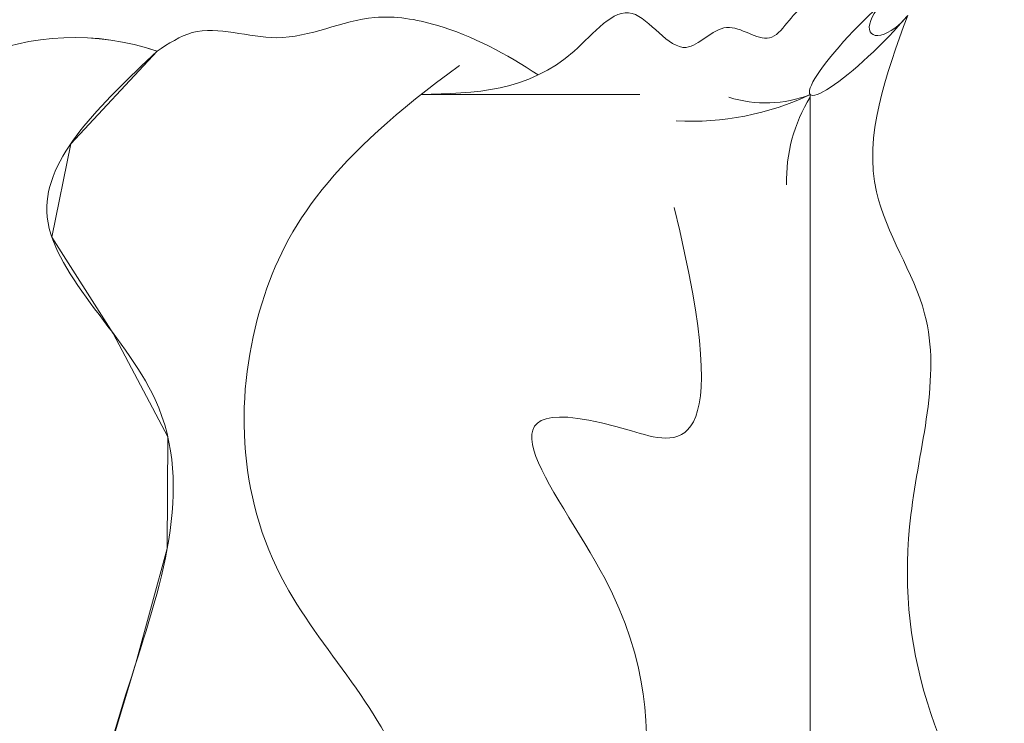
# Model space of a CAD drawing. Units: inches. Extents: x 2083 to 3317, y 1141 to 2115.
# Tile 10 of 256: x 2278 to 2324, y 1329 to 1361. Entities that reach past the tile are written whole.
import ezdxf

# ---------------------------------------------------------------- set-up
doc = ezdxf.new("R2010")
doc.units = ezdxf.units.IN
for name, color, linetype, lineweight in [('A-ANNO-DIMS', 2, 'Continuous', 18), ('A-FURN', 8, 'Continuous', 18), ('www.cadblocksfree.com', 7, 'Continuous', 9)]:
    doc.layers.add(name, color=color, linetype=linetype, lineweight=lineweight)
doc.layers.add('A-WALL-PATT', color=251, linetype='Continuous', lineweight=13, true_color=0x636466)
doc.styles.get("Standard").update_dxf_attribs({"font": 'arial.ttf'})
doc.dimstyles.new('ISO-25', dxfattribs={"dimtxt": 12, "dimasz": 12, "dimexe": 1.25, "dimexo": 0.625, "dimtad": 1, "dimlunit": 3, "dimtxsty": 'Standard', "dimcen": 2.5, "dimadec": 0, "dimazin": 0, "dimtfac": 1, "dimtmove": 0, "dimatfit": 3, "dimfxl": 1, "dimarcsym": 0})

# ---------------------------------------------------------------- blocks, each defined once
blk = doc.blocks.new('bed')
at = {"layer": 'www.cadblocksfree.com', "ltscale": 0.2}
for p, q in [((3426.379, 1399.908), (3426.379, 1410.814)), ((3363.387, 1391.414), (3426.379, 1391.414))]:
    blk.add_line(p, q, dxfattribs=at)
for centre, radius, start, end in [((3416.575, 1428.082), 12.646, 341.0268, 23.7782), ((3438.819, 1397.314), 13.768, 176.7525, 205.373), ((3432.135, 1393.639), 6.173, 162.6475, 201.1361), ((3422.111, 1384.801), 7.798, 58.0013, 91.6551)]:
    blk.add_arc(centre, radius, start, end, dxfattribs=at)
for centre, major_axis, ratio, start_param, end_param in [((3429.422, 1388.371), (-3.043, 3.043), 0.168252, 4.250342, 8.316029), ((3430.477, 1387.316), (-1.055, 1.055), 0.453532, 4.422107, 8.144264)]:
    blk.add_ellipse(centre, major_axis=major_axis, ratio=ratio, start_param=start_param, end_param=end_param, dxfattribs=at)
for points, knots in [([(3365.512, 1424.213), (3370.519, 1427.004), (3381.149, 1429.825), (3396.214, 1425.866), (3410.541, 1420.654), (3420.273, 1432.695), (3425.882, 1426.771), (3428.534, 1423.97)], [0.099185, 0.099185, 0.099185, 0.099185, 0.523647, 0.927087, 1.289918, 1.564439, 1.810555, 1.810555, 1.810555, 1.810555]), ([(3428.534, 1423.97), (3428.914, 1423.397), (3430.098, 1421.613), (3428.491, 1417.656), (3430.593, 1413.794), (3429.801, 1409.122), (3428.396, 1406.564), (3427.355, 1404.971)], [0, 0, 0, 0, 0.050513, 0.157399, 0.2842023, 0.3628173, 0.5066917, 0.5066917, 0.5066917, 0.5066917]), ([(3362.057, 1409.866), (3363.638, 1413.65), (3372.978, 1421.337), (3389.682, 1406.045), (3402.396, 1419.984), (3416.037, 1420.167), (3423.233, 1415.231), (3427.827, 1408.899)], [0.029901, 0.029901, 0.029901, 0.029901, 0.276967, 0.797115, 1.093669, 1.464666, 1.788489, 1.788489, 1.788489, 1.788489]), ([(3431.237, 1387.473), (3430.882, 1388.172), (3430.205, 1389.505), (3431.478, 1391.985), (3428.294, 1393.194), (3430.501, 1395.689), (3427.558, 1397.866), (3431.841, 1400.386), (3426.535, 1404.33), (3426.443, 1408.152), (3426.379, 1410.814)], [0, 0, 0, 0, 2.267059, 4.324559, 6.685584, 8.878641, 11.121502, 14.300359, 17.755284, 25.682856, 25.682856, 25.682856, 25.682856]), ([(3368.632, 1397.839), (3375.978, 1400.489), (3385.349, 1402.757), (3397.531, 1395.273), (3413.593, 1410.377), (3407.806, 1395.019), (3420.759, 1398.2)], [0.029901, 0.029901, 0.029901, 0.029901, 0.276967, 0.797115, 1.093669, 1.16836, 1.16836, 1.16836, 1.16836]), ([(3430.32, 1386.556), (3427.327, 1387.653), (3422.148, 1389.55), (3414.529, 1384.137), (3405.607, 1387.046), (3396.29, 1386.314), (3386.838, 1381.282), (3377.742, 1390.272), (3370.778, 1384.799), (3364.626, 1383.966), (3363.275, 1388.265), (3360.778, 1387.151), (3359.446, 1386.556)], [0, 0, 0, 0, 8.93042, 15.449194, 25.485629, 34.878505, 43.598887, 54.554403, 64.16647, 67.461673, 70.610457, 74.213583, 74.213583, 74.213583, 74.213583])]:
    blk.add_open_spline(points, degree=3, knots=knots, dxfattribs=at)
blk = doc.blocks.new('*D22')
at = {"layer": 'A-ANNO-DIMS', "color": 0, "lineweight": -2, "transparency": 16777216}
for p, q in [((2235.96, 1362.739), (2235.96, 1376.309)), ((2322.26, 1362.739), (2322.26, 1376.309)), ((2235.96, 1375.059), (2083.007, 1375.059)), ((2310.26, 1375.059), (2247.96, 1375.059))]:
    blk.add_line(p, q, dxfattribs=at)
at = {"layer": 'A-ANNO-DIMS', "color": 0, "transparency": 16777216}
for points in [[(2247.96, 1377.059), (2247.96, 1373.059), (2235.96, 1375.059)], [(2310.26, 1377.059), (2310.26, 1373.059), (2322.26, 1375.059)]]:
    blk.add_solid(points, dxfattribs=at)
at = {"layer": 'Defpoints', "color": 0, "transparency": 16777216}
for p in [(2235.96, 1375.059), (2235.96, 1362.114), (2322.26, 1362.114)]:
    blk.add_point(p, dxfattribs=at)
at = {"layer": 'A-ANNO-DIMS', "color": 0, "transparency": 16777216, "insert": (2153.483, 1381.889), "char_height": 12, "attachment_point": 5}
blk.add_mtext('BED 7\'-2 1/2" TYP.', dxfattribs=at)
blk = doc.blocks.new('*D23')
at = {"layer": 'A-ANNO-DIMS', "color": 0, "lineweight": -2, "transparency": 16777216}
for p, q in [((2335.205, 1362.114), (2335.205, 1476.472)), ((2322.885, 1362.114), (2336.455, 1362.114)), ((2335.205, 1306.473), (2335.205, 1350.114)), ((2322.885, 1294.473), (2336.455, 1294.473))]:
    blk.add_line(p, q, dxfattribs=at)
at = {"layer": 'A-ANNO-DIMS', "color": 0, "transparency": 16777216}
for points in [[(2333.205, 1350.114), (2337.205, 1350.114), (2335.205, 1362.114)], [(2333.205, 1306.473), (2337.205, 1306.473), (2335.205, 1294.473)]]:
    blk.add_solid(points, dxfattribs=at)
at = {"layer": 'Defpoints', "color": 0, "transparency": 16777216}
for p in [(2322.26, 1362.114), (2335.205, 1362.114), (2322.26, 1294.473)]:
    blk.add_point(p, dxfattribs=at)
at = {"layer": 'A-ANNO-DIMS', "color": 0, "transparency": 16777216, "insert": (2328.376, 1425.293), "char_height": 12, "attachment_point": 5, "rotation": 90}
blk.add_mtext('5\'-7 1/2" TYP.', dxfattribs=at)

msp = doc.modelspace()

# ---------------------------------------------------------------- hatches: boundary and pattern name
at = {"layer": 'A-WALL-PATT'}
h = msp.add_hatch(color=256, dxfattribs=at)
h.dxf.hatch_style = 1
h.paths.add_polyline_path([(3126.96, 2020.761), (2748.96, 2020.761), (2604.96, 2020.761), (2226.96, 2020.761), (2226.96, 1702.761), (2466.96, 1702.761), (2466.96, 1582.761), (2418.96, 1582.761), (2418.96, 1477.761), (2226.96, 1477.761), (2226.96, 1263.261), (2544.96, 1263.261), (2544.96, 1411.761), (2604.96, 1411.761), (2685.96, 1411.761), (2685.96, 1420.761), (2604.96, 1420.761), (2604.96, 1573.761), (2604.96, 1702.761), (2604.96, 2011.761), (2748.96, 2011.761), (2748.96, 1702.761), (2862.96, 1702.761), (2862.96, 1621.761), (2871.96, 1621.761), (2871.96, 1702.761), (2883.96, 1702.761), (2883.96, 1706.939, -0.026459), (2883.96, 1711.761), (2757.96, 1711.761), (2757.96, 1807.761), (2787.96, 1807.761), (2787.96, 1812.261), (2757.96, 1812.261), (2757.96, 2011.761), (2877.96, 2011.761), (2877.96, 1812.261), (2847.96, 1812.261), (2847.96, 1807.761), (2889.836, 1807.761), (2889.836, 1812.261), (2882.46, 1812.261), (2882.46, 2011.761), (3117.96, 2011.761), (3117.96, 1812.261), (2937.836, 1812.261), (2937.836, 1807.761), (2995.71, 1807.761), (2995.71, 1796.118), (3000.21, 1796.118), (3000.21, 1807.761), (3117.96, 1807.761), (3117.96, 1711.761), (3000.21, 1711.761), (3000.21, 1760.118), (2998.573, 1760.118, -0.020711), (2995.71, 1760.118), (2995.71, 1711.761), (2931.96, 1711.761), (2931.96, 1702.761), (3126.96, 1702.761)])
h.paths.add_polyline_path([(2471.46, 2011.761), (2471.46, 1810.011), (2462.717, 1810.011), (2462.717, 1805.511), (2505.96, 1805.511), (2505.96, 1810.011), (2475.96, 1810.011), (2475.96, 2011.761), (2595.96, 2011.761), (2595.96, 1810.011), (2565.96, 1810.011), (2565.96, 1805.511), (2595.96, 1805.511), (2595.96, 1711.761), (2235.96, 1711.761), (2235.96, 1805.511), (2353.71, 1805.511), (2353.71, 1796.054), (2358.21, 1796.054), (2358.21, 1805.511), (2414.717, 1805.511), (2414.717, 1810.011), (2235.96, 1810.011), (2235.96, 2011.761)], flags=16)
h.paths.add_polyline_path([(2270.205, 1994.61), (2270.205, 1970.61), (2246.205, 1970.61), (2246.205, 1994.61)], flags=0)
edge = h.paths.add_edge_path(flags=0)
edge.add_ellipse((2332.027, 1899.798), major_axis=(-3.043, 3.043), ratio=0.168252, start_angle=-161.3322, end_angle=-156.3071, ccw=False)
edge.add_ellipse((2333.082, 1898.744), major_axis=(-1.055, 1.055), ratio=0.453532, start_angle=-123.371, end_angle=-94.1591)
edge = h.paths.add_edge_path(flags=0)
edge.add_ellipse((2332.027, 1968.876), major_axis=(3.043, 3.043), ratio=0.168252, start_angle=18.6678, end_angle=23.6929)
edge.add_spline(control_points=[(2332.926, 1970.691), (2332.227, 1970.336), (2330.894, 1969.659), (2328.413, 1970.932), (2327.204, 1967.749), (2324.71, 1969.956), (2322.533, 1967.012), (2320.013, 1971.296), (2317.68, 1968.158), (2316.041, 1967.102), (2315.427, 1966.81)], knot_values=[0, 0, 0, 0, 2.267059, 4.324559, 6.685584, 8.878641, 11.121502, 14.300359, 17.755284, 19.732645, 19.732645, 19.732645, 19.732645], degree=3, periodic=0)
edge.add_ellipse((2332.027, 1968.876), major_axis=(3.043, 3.043), ratio=0.168252, start_angle=18.6678, end_angle=23.6929, ccw=False)
edge.add_ellipse((2333.082, 1969.931), major_axis=(1.055, 1.055), ratio=0.453532, start_angle=56.629, end_angle=85.8409, ccw=False)
edge = h.paths.add_edge_path(flags=0)
edge.add_spline(control_points=[(2296.428, 1967.988), (2293.628, 1965.336), (2287.704, 1959.727), (2299.744, 1949.996), (2294.533, 1935.669), (2290.573, 1920.604), (2293.394, 1909.974), (2296.185, 1904.967)], knot_values=[0.099185, 0.099185, 0.099185, 0.099185, 0.345301, 0.619822, 0.982653, 1.386093, 1.810555, 1.810555, 1.810555, 1.810555], degree=3, periodic=0)
edge.add_spline(control_points=[(2296.185, 1904.967), (2297.384, 1902.619), (2298.001, 1901.949), (2298.553, 1901.468)], knot_values=[0.006246, 0.006246, 0.006246, 0.006246, 0.055476, 0.055476, 0.055476, 0.055476], degree=3, periodic=0)
edge.add_spline(control_points=[(2298.553, 1901.468), (2297.259, 1900.923), (2295.225, 1900.232), (2293.06, 1900.614), (2292.101, 1900.788), (2292.09, 1900.791)], knot_values=[0.312835, 0.312835, 0.312835, 0.312835, 0.40178, 0.474987, 0.475903, 0.475903, 0.475903, 0.475903], degree=3, periodic=0)
edge.add_arc((2292.794, 1904.664), 3.937, 215.4209, 259.6982, ccw=False)
edge.add_spline(control_points=[(2289.585, 1902.382), (2289.477, 1902.535), (2289.368, 1902.688), (2289.261, 1902.841)], knot_values=[0.102872, 0.102872, 0.102872, 0.102872, 0.116896, 0.116896, 0.116896, 0.116896], degree=3, periodic=0)
edge.add_spline(control_points=[(2289.261, 1902.841), (2288.687, 1902.55), (2287.64, 1902.02), (2285.881, 1901.874), (2283.853, 1901.504), (2281.72, 1899.711), (2278.467, 1899.493), (2276.157, 1901.883), (2272.259, 1899.804), (2267.778, 1901.843), (2262.244, 1900.184), (2257.415, 1901.782), (2254.318, 1900.726), (2253.178, 1900.337)], knot_values=[0, 0, 0, 0, 1.907977, 3.477176, 5.261074, 7.972851, 11.680248, 13.717921, 16.939592, 22.789562, 27.502503, 33.595215, 37.145618, 37.145618, 37.145618, 37.145618], degree=3, periodic=0)
edge.add_line((2253.178, 1900.337), (2250.244, 1902.841))
edge.add_line((2250.244, 1902.841), (2250.244, 1965.833))
edge.add_line((2250.244, 1965.833), (2253.178, 1968.337))
edge.add_spline(control_points=[(2253.178, 1968.337), (2254.318, 1967.948), (2257.415, 1966.892), (2262.244, 1968.49), (2267.778, 1966.831), (2271.527, 1968.537), (2273.876, 1967.828), (2274.207, 1967.728)], knot_values=[0, 0, 0, 0, 0.09018, 0.244935, 0.364644, 0.513233, 0.537855, 0.537855, 0.537855, 0.537855], degree=3, periodic=0)
edge.add_arc((2274.353, 1963.793), 3.937, 72.0511, 92.1279, ccw=False)
edge.add_arc((2281.297, 1985.23), 18.596, 252.0511, 288.5657)
edge.add_arc((2292.317, 1956.029), 12.646, 71.0268, 113.7782, ccw=False)
edge = h.paths.add_edge_path(flags=0)
edge.add_spline(control_points=[(2274.899, 1951.856), (2275.066, 1951.617), (2275.233, 1951.377), (2275.398, 1951.136)], knot_values=[1.409916, 1.409916, 1.409916, 1.409916, 1.43159, 1.43159, 1.43159, 1.43159], degree=3, periodic=0)
edge.add_spline(control_points=[(2275.398, 1951.136), (2275.792, 1950.562), (2276.179, 1949.984), (2276.546, 1949.397)], knot_values=[1.358238, 1.358238, 1.358238, 1.358238, 1.409916, 1.409916, 1.409916, 1.409916], degree=3, periodic=0)
edge.add_line((2276.546, 1949.397), (2277.437, 1947.862))
edge.add_spline(control_points=[(2277.437, 1947.862), (2276.304, 1945.673), (2274.64, 1942.427), (2274.632, 1938.094), (2272.799, 1930.852), (2274.356, 1943.897), (2275.948, 1947.923), (2276.546, 1949.397)], knot_values=[0.005632, 0.005632, 0.005632, 0.005632, 0.186014, 0.266002, 0.357087, 0.59639, 0.739732, 0.739732, 0.739732, 0.739732], degree=3, periodic=0)
edge.add_spline(control_points=[(2276.546, 1949.397), (2276.179, 1949.984), (2275.792, 1950.562), (2275.398, 1951.136)], knot_values=[1.358238, 1.358238, 1.358238, 1.358238, 1.409916, 1.409916, 1.409916, 1.409916], degree=3, periodic=0)
edge.add_spline(control_points=[(2275.398, 1951.136), (2274.943, 1950.08), (2274.208, 1948.025), (2273.935, 1944.851), (2272.469, 1937.627), (2273.466, 1945.696), (2274.701, 1951.059), (2274.899, 1951.856)], knot_values=[0.104364, 0.104364, 0.104364, 0.104364, 0.189636, 0.269624, 0.36071, 0.600013, 0.644622, 0.644622, 0.644622, 0.644622], degree=3, periodic=0)
h.paths.add_polyline_path([(2269.168, 1963.128, -0.357527), (2268.171, 1960.976, -0.092561), (2268.171, 1939.436, -0.357527), (2269.168, 1937.285, -0.357527), (2267.016, 1938.282, -0.164785), (2254.686, 1938.282, -0.357527), (2252.534, 1937.285, -0.357527), (2253.531, 1939.436, -0.092561), (2253.531, 1960.976, -0.357527), (2252.534, 1963.128, -0.357527), (2254.686, 1962.131, -0.164785), (2267.016, 1962.131, -0.357527)], flags=0)
h.paths.add_polyline_path([(2248.874, 1967.802), (2248.874, 1957.028), (2249.458, 1957.028), (2249.458, 1911.647), (2248.874, 1911.647), (2248.874, 1900.873), (2246.512, 1900.873, 0.197327), (2244.15, 1902.457), (2244.15, 1966.218, 0.197327), (2246.512, 1967.802)], flags=0)
h.paths.add_polyline_path([(2269.168, 1931.389, -0.357527), (2268.171, 1929.238, -0.092561), (2268.171, 1907.698, -0.357527), (2269.168, 1905.547, -0.357527), (2267.016, 1906.544, -0.164785), (2254.686, 1906.544, -0.357527), (2252.534, 1905.547, -0.357527), (2253.531, 1907.698, -0.092561), (2253.531, 1929.238, -0.357527), (2252.534, 1931.389, -0.357527), (2254.686, 1930.392, -0.164785), (2267.016, 1930.392, -0.357527)], flags=0)
edge = h.paths.add_edge_path(flags=0)
edge.add_spline(control_points=[(2276.197, 1906.724), (2276.168, 1909.029), (2276.114, 1913.372), (2270.598, 1924.925), (2273.905, 1919.013), (2275.922, 1916.262), (2275.475, 1912.402), (2277.258, 1910.381), (2276.696, 1908.225), (2276.646, 1906.813), (2276.618, 1906.008)], knot_values=[0, 0, 0, 0, 8.61026, 16.221274, 18.843057, 23.804898, 27.440828, 29.356102, 31.203478, 33.650687, 33.650687, 33.650687, 33.650687], degree=3, periodic=0)
edge.add_spline(control_points=[(2276.618, 1906.008), (2276.623, 1905.624), (2276.498, 1904.629), (2275.442, 1903.855), (2274.937, 1903.08), (2274.859, 1902.841)], knot_values=[0.156488, 0.156488, 0.156488, 0.156488, 0.184398, 0.231376, 0.250598, 0.250598, 0.250598, 0.250598], degree=3, periodic=0)
edge.add_line((2274.859, 1902.841), (2276.506, 1902.841))
edge.add_spline(control_points=[(2276.506, 1902.841), (2276.788, 1903.085), (2277.665, 1904.125), (2278.25, 1904.341), (2277.654, 1908.527), (2278.156, 1906.228), (2278.1, 1905.286), (2278.847, 1904.069), (2277.857, 1903.415), (2277.874, 1902.991), (2277.904, 1902.841)], knot_values=[0.059574, 0.059574, 0.059574, 0.059574, 0.080753, 0.103741, 0.16972, 0.176036, 0.207137, 0.240474, 0.262341, 0.27366, 0.27366, 0.27366, 0.27366], degree=3, periodic=0)
edge.add_line((2277.904, 1902.841), (2280.03, 1902.841))
edge.add_spline(control_points=[(2280.03, 1902.841), (2279.888, 1903.088), (2279.499, 1903.982), (2280.152, 1905.939), (2278.104, 1909.658), (2279.762, 1907.185), (2280.328, 1904.875), (2280.485, 1903.49), (2281.463, 1903.249), (2281.758, 1902.936), (2281.834, 1902.841)], knot_values=[0.013856, 0.013856, 0.013856, 0.013856, 0.034874, 0.088867, 0.107879, 0.126738, 0.158714, 0.193757, 0.217487, 0.226722, 0.226722, 0.226722, 0.226722], degree=3, periodic=0)
edge.add_spline(control_points=[(2281.834, 1902.841), (2281.788, 1902.827), (2281.647, 1902.783), (2281.396, 1902.859), (2281.088, 1902.985), (2280.721, 1903.061), (2280.333, 1903.026), (2280.125, 1902.899), (2280.03, 1902.841)], knot_values=[0, 0, 0, 0, 0.14413, 0.435517, 0.749276, 1.153046, 1.548371, 1.878348, 1.878348, 1.878348, 1.878348], degree=3, periodic=0)
edge.add_line((2280.03, 1902.841), (2277.904, 1902.841))
edge.add_spline(control_points=[(2277.904, 1902.841), (2277.893, 1902.796), (2277.865, 1902.68), (2277.607, 1902.687), (2277.274, 1902.801), (2276.838, 1902.62), (2276.584, 1902.789), (2276.506, 1902.841)], knot_values=[0, 0, 0, 0, 0.127189, 0.326199, 0.628009, 1.24357, 1.515331, 1.515331, 1.515331, 1.515331], degree=3, periodic=0)
edge.add_line((2276.506, 1902.841), (2274.859, 1902.841))
edge.add_spline(control_points=[(2274.859, 1902.841), (2274.814, 1902.899), (2274.725, 1903.013), (2274.493, 1903.119), (2274.244, 1902.961), (2273.937, 1903.185), (2273.614, 1902.983), (2273.408, 1902.883), (2273.322, 1902.841)], knot_values=[0, 0, 0, 0, 0.21843, 0.436957, 0.687977, 0.990379, 1.398396, 1.69185, 1.69185, 1.69185, 1.69185], degree=3, periodic=0)
edge.add_spline(control_points=[(2273.322, 1902.841), (2273.617, 1903.446), (2274.274, 1904.538), (2276.027, 1904.574), (2276.207, 1906.584), (2276.197, 1906.724)], knot_values=[0.012227, 0.012227, 0.012227, 0.012227, 0.059472, 0.106218, 0.134458, 0.134458, 0.134458, 0.134458], degree=3, periodic=0)
h.paths.add_polyline_path([(2270.776, 1897.79), (2270.776, 1873.79), (2246.776, 1873.79), (2246.776, 1897.79)], flags=0)
h.paths.add_polyline_path([(2353.71, 1760.005), (2353.71, 1760.054), (2358.21, 1760.054, -0.033729)], flags=0)
h.paths.add_polyline_path([(2321.819, 1737.529), (2341.995, 1737.529, -0.414214), (2343.203, 1736.321), (2343.203, 1721.021, -0.414214), (2341.995, 1719.813), (2321.819, 1719.813, -0.414214), (2320.611, 1721.021), (2320.611, 1736.321, -0.414214)], flags=0)
h.paths.add_polyline_path([(2324.235, 1736.321), (2339.579, 1736.321, -0.414214), (2341.995, 1733.905), (2341.995, 1725.45, -0.414214), (2339.579, 1723.034), (2333.681, 1723.034), (2333.845, 1722.045, -0.870646), (2335.425, 1721.826, -0.767327), (2333.923, 1721.423), (2331.291, 1721.423, -0.767327), (2329.788, 1721.826, -0.870646), (2331.368, 1722.045), (2331.533, 1723.034), (2324.235, 1723.034, -0.414214), (2321.819, 1725.45), (2321.819, 1733.905, -0.414214)], flags=0)
h.paths.add_polyline_path([(2570.484, 1928.615), (2589.684, 1928.615), (2590.169, 1928.615), (2590.169, 1904.993), (2570.484, 1904.993)], flags=0)
h.paths.add_polyline_path([(2574.447, 1927.264, -1), (2572.829, 1927.264, -1)], flags=0)
h.paths.add_polyline_path([(2573.09, 1926.941), (2573.925, 1927.776), (2574.148, 1927.553), (2573.313, 1926.718)], flags=0)
h.paths.add_polyline_path([(2578.779, 1919.73, -1), (2571.592, 1919.73, -1)], flags=0)
h.paths.add_polyline_path([(2578.385, 1919.73, -1), (2571.985, 1919.73, -1)], flags=0)
h.paths.add_polyline_path([(2331.596, 1729.476, -1), (2333.618, 1729.476, -1)], flags=0)
h.paths.add_polyline_path([(2578.034, 1927.264, -1), (2576.416, 1927.264, -1)], flags=0)
h.paths.add_polyline_path([(2576.689, 1927.531), (2576.912, 1927.754), (2577.747, 1926.919), (2577.524, 1926.696)], flags=0)
h.paths.add_polyline_path([(2578.139, 1909.86, -1), (2572.232, 1909.86, -1)], flags=0)
h.paths.add_polyline_path([(2577.745, 1909.86, -1), (2572.625, 1909.86, -1)], flags=0)
h.paths.add_polyline_path([(2583.798, 1927.264, -1), (2582.179, 1927.264, -1)], flags=0)
h.paths.add_polyline_path([(2582.719, 1927.754), (2583.554, 1926.919), (2583.331, 1926.696), (2582.496, 1927.531)], flags=0)
h.paths.add_polyline_path([(2582.496, 1927.531), (2582.719, 1927.754), (2583.554, 1926.919), (2583.331, 1926.696)], flags=0)
h.paths.add_polyline_path([(2587.739, 1920.53, -1), (2581.832, 1920.53, -1)], flags=0)
h.paths.add_polyline_path([(2587.345, 1920.53, -1), (2582.225, 1920.53, -1)], flags=0)
h.paths.add_polyline_path([(2587.385, 1927.264, -1), (2585.766, 1927.264, -1)], flags=0)
h.paths.add_polyline_path([(2586.082, 1926.98), (2586.917, 1927.815), (2587.14, 1927.593), (2586.305, 1926.758)], flags=0)
h.paths.add_polyline_path([(2588.379, 1910.66, -1), (2581.192, 1910.66, -1)], flags=0)
h.paths.add_polyline_path([(2587.985, 1910.66, -1), (2581.585, 1910.66, -1)], flags=0)
h.paths.add_polyline_path([(2417.168, 1729.478), (2437.344, 1729.478, -0.414214), (2438.552, 1728.27), (2438.552, 1712.969, -0.414214), (2437.344, 1711.761), (2417.168, 1711.761, -0.414214), (2415.96, 1712.969), (2415.96, 1728.27, -0.414214)], flags=0)
h.paths.add_polyline_path([(2419.584, 1728.27), (2434.928, 1728.27, -0.414214), (2437.344, 1725.854), (2437.344, 1717.398, -0.414214), (2434.928, 1714.983), (2429.029, 1714.983), (2429.194, 1713.994, -0.870646), (2430.774, 1713.775, -0.767327), (2429.271, 1713.372), (2426.64, 1713.372, -0.767327), (2425.137, 1713.775, -0.870646), (2426.717, 1713.994), (2426.882, 1714.983), (2419.584, 1714.983, -0.414214), (2417.168, 1717.398), (2417.168, 1725.854, -0.414214)], flags=0)
h.paths.add_polyline_path([(2419.584, 1728.27), (2434.928, 1728.27, -0.414214), (2437.344, 1725.854), (2437.344, 1717.398, -0.414214), (2434.928, 1714.983), (2429.029, 1714.983), (2428.358, 1719.009), (2427.553, 1719.009), (2426.882, 1714.983), (2419.584, 1714.983, -0.414214), (2417.168, 1717.398), (2417.168, 1725.854, -0.414214)], flags=0)
h.paths.add_polyline_path([(2426.944, 1721.425, -1), (2428.967, 1721.425, -1)], flags=0)
h.paths.add_polyline_path([(2475.96, 1702.761), (2595.96, 1702.761), (2595.96, 1582.761), (2475.96, 1582.761)], flags=16)
h.paths.add_polyline_path([(2427.96, 1573.761), (2595.96, 1573.761), (2595.96, 1468.761), (2595.96, 1420.761), (2384.46, 1420.761), (2384.46, 1468.761), (2427.96, 1468.761)], flags=16)
h.paths.add_polyline_path([(2379.96, 1468.761), (2379.96, 1420.761), (2235.96, 1420.761), (2235.96, 1468.761)], flags=16)
h.paths.add_polyline_path([(2317.816, 1466.696), (2337.992, 1466.696, -0.414214), (2339.2, 1465.488), (2339.2, 1450.187, -0.414214), (2337.992, 1448.979), (2317.816, 1448.979, -0.414214), (2316.608, 1450.187), (2316.608, 1465.488, -0.414214)], flags=0)
h.paths.add_polyline_path([(2320.232, 1465.488), (2335.576, 1465.488, -0.414214), (2337.992, 1463.072), (2337.992, 1454.616, -0.414214), (2335.576, 1452.2), (2329.677, 1452.2), (2329.842, 1451.212, -0.870646), (2331.422, 1450.992, -0.767327), (2329.92, 1450.59), (2327.288, 1450.59, -0.767327), (2325.785, 1450.992, -0.870646), (2327.365, 1451.212), (2327.53, 1452.2), (2320.232, 1452.2, -0.414214), (2317.816, 1454.616), (2317.816, 1463.072, -0.414214)], flags=0)
h.paths.add_polyline_path([(2320.232, 1465.488), (2335.576, 1465.488, -0.414214), (2337.992, 1463.072), (2337.992, 1454.616, -0.414214), (2335.576, 1452.2), (2329.677, 1452.2), (2329.006, 1456.227), (2328.201, 1456.227), (2327.53, 1452.2), (2320.232, 1452.2, -0.414214), (2317.816, 1454.616), (2317.816, 1463.072, -0.414214)], flags=0)
h.paths.add_polyline_path([(2327.593, 1458.643, -1), (2329.615, 1458.643, -1)], flags=0)
h.paths.add_polyline_path([(2244.412, 1433.34), (2241.921, 1433.34, -0.414214), (2240.018, 1435.244), (2240.018, 1440.953, -0.414211), (2241.921, 1442.856), (2244.412, 1442.856, -1.976472)], flags=0)
h.paths.add_polyline_path([(2245.357, 1434.398, -0.414214), (2245.357, 1441.799, -2.144098)], flags=0)
h.paths.add_polyline_path([(2535.96, 1416.261), (2535.96, 1272.261), (2235.96, 1272.261), (2235.96, 1416.261)], flags=16)
h.paths.add_polyline_path([(2260.12, 1384.293), (2260.12, 1362.039), (2237.865, 1362.039), (2237.865, 1384.293)], flags=0)
edge = h.paths.add_edge_path(flags=0)
edge.add_line((2318.252, 1362.093), (2318.146, 1362.001))
edge.add_ellipse((2317.445, 1360.431), major_axis=(2.822, 2.822), ratio=0.168252, start_angle=18.6678, end_angle=20.9481, ccw=False)
edge.add_ellipse((2318.423, 1361.409), major_axis=(0.978, 0.978), ratio=0.453532, start_angle=56.629, end_angle=70.2262, ccw=False)
edge = h.paths.add_edge_path(flags=0)
edge.add_line((2319.107, 1295.571), (2319.015, 1295.677))
edge.add_ellipse((2317.445, 1296.378), major_axis=(-2.822, 2.822), ratio=0.168252, start_angle=-161.3322, end_angle=-159.0519, ccw=False)
edge.add_ellipse((2318.423, 1295.4), major_axis=(-0.978, 0.978), ratio=0.453532, start_angle=-123.371, end_angle=-109.7738)
edge = h.paths.add_edge_path(flags=0)
edge.add_spline(control_points=[(2284.21, 1301.17), (2284.581, 1300.445), (2284.891, 1299.892), (2285.16, 1299.461)], knot_values=[0.039066, 0.039066, 0.039066, 0.039066, 0.055476, 0.055476, 0.055476, 0.055476], degree=3, periodic=0)
edge.add_line((2285.16, 1299.461), (2284.21, 1301.17))
edge = h.paths.add_edge_path(flags=0)
edge.add_line((2280.412, 1297.298), (2283.37, 1297.036))
edge.add_line((2283.37, 1297.036), (2286.406, 1297.926))
edge.add_spline(control_points=[(2286.406, 1297.926), (2285.305, 1297.463), (2284.345, 1297.129), (2283.37, 1297.036)], knot_values=[0.394369, 0.394369, 0.394369, 0.394369, 0.475903, 0.475903, 0.475903, 0.475903], degree=3, periodic=0)
edge.add_spline(control_points=[(2283.37, 1297.036), (2283.281, 1297.028), (2282.316, 1296.957), (2281.313, 1297.134), (2280.423, 1297.296), (2280.412, 1297.298)], knot_values=[0.312835, 0.312835, 0.312835, 0.312835, 0.320246, 0.393453, 0.394369, 0.394369, 0.394369, 0.394369], degree=3, periodic=0)
edge = h.paths.add_edge_path(flags=0)
edge.add_line((2284.436, 1359.607), (2280.446, 1355.328))
edge.add_line((2280.446, 1355.328), (2279.58, 1351.018))
edge.add_line((2279.58, 1351.018), (2282.413, 1346.58))
edge.add_spline(control_points=[(2282.413, 1346.58), (2283.153, 1345.589), (2284.253, 1344.029), (2284.801, 1342.387), (2284.935, 1341.806)], knot_values=[1.240098, 1.240098, 1.240098, 1.240098, 1.332892, 1.382712, 1.382712, 1.382712, 1.382712], degree=3, periodic=0)
edge.add_spline(control_points=[(2284.935, 1341.806), (2285.319, 1340.141), (2285.233, 1338.409), (2284.91, 1336.654)], knot_values=[1.097484, 1.097484, 1.097484, 1.097484, 1.240098, 1.240098, 1.240098, 1.240098], degree=3, periodic=0)
edge.add_spline(control_points=[(2284.91, 1336.654), (2284.587, 1334.899), (2284.027, 1333.12), (2283.463, 1331.361)], knot_values=[0.95487, 0.95487, 0.95487, 0.95487, 1.097484, 1.097484, 1.097484, 1.097484], degree=3, periodic=0)
edge.add_line((2283.463, 1331.361), (2281.89, 1326.153))
edge.add_line((2281.89, 1326.153), (2280.756, 1321.056))
edge.add_line((2280.756, 1321.056), (2280.299, 1316.002))
edge.add_line((2280.299, 1316.002), (2280.716, 1310.95))
edge.add_line((2280.716, 1310.95), (2282.028, 1305.972))
edge.add_line((2282.028, 1305.972), (2284.21, 1301.17))
edge.add_spline(control_points=[(2284.21, 1301.17), (2283.341, 1302.73), (2282.612, 1304.336), (2282.028, 1305.972)], knot_values=[0.099185, 0.099185, 0.099185, 0.099185, 0.241799, 0.241799, 0.241799, 0.241799], degree=3, periodic=0)
edge.add_spline(control_points=[(2282.028, 1305.972), (2281.444, 1307.608), (2281.005, 1309.273), (2280.716, 1310.95)], knot_values=[0.241799, 0.241799, 0.241799, 0.241799, 0.384413, 0.384413, 0.384413, 0.384413], degree=3, periodic=0)
edge.add_spline(control_points=[(2280.716, 1310.95), (2280.433, 1312.588), (2280.289, 1314.277), (2280.299, 1315.962), (2280.299, 1316.002)], knot_values=[0.384413, 0.384413, 0.384413, 0.384413, 0.523647, 0.527028, 0.527028, 0.527028, 0.527028], degree=3, periodic=0)
edge.add_spline(control_points=[(2280.299, 1316.002), (2280.312, 1317.687), (2280.478, 1319.368), (2280.756, 1321.056)], knot_values=[0.527028, 0.527028, 0.527028, 0.527028, 0.669642, 0.669642, 0.669642, 0.669642], degree=3, periodic=0)
edge.add_spline(control_points=[(2280.756, 1321.056), (2281.035, 1322.744), (2281.426, 1324.44), (2281.89, 1326.153)], knot_values=[0.669642, 0.669642, 0.669642, 0.669642, 0.812256, 0.812256, 0.812256, 0.812256], degree=3, periodic=0)
edge.add_spline(control_points=[(2281.89, 1326.153), (2282.264, 1327.533), (2282.788, 1329.262), (2283.353, 1331.018), (2283.463, 1331.361)], knot_values=[0.812256, 0.812256, 0.812256, 0.812256, 0.927087, 0.95487, 0.95487, 0.95487, 0.95487], degree=3, periodic=0)
edge.add_line((2283.463, 1331.361), (2284.91, 1336.654))
edge.add_line((2284.91, 1336.654), (2284.935, 1341.806))
edge.add_line((2284.935, 1341.806), (2282.413, 1346.58))
edge.add_spline(control_points=[(2282.413, 1346.58), (2281.275, 1348.104), (2280.078, 1349.57), (2279.58, 1351.018)], knot_values=[1.382712, 1.382712, 1.382712, 1.382712, 1.525326, 1.525326, 1.525326, 1.525326], degree=3, periodic=0)
edge.add_spline(control_points=[(2279.58, 1351.018), (2279.443, 1351.415), (2279.136, 1352.857), (2279.735, 1354.29), (2280.446, 1355.328)], knot_values=[1.525326, 1.525326, 1.525326, 1.525326, 1.564439, 1.667941, 1.667941, 1.667941, 1.667941], degree=3, periodic=0)
edge.add_spline(control_points=[(2280.446, 1355.328), (2281.426, 1356.758), (2282.931, 1358.183), (2284.436, 1359.607)], knot_values=[1.667941, 1.667941, 1.667941, 1.667941, 1.810555, 1.810555, 1.810555, 1.810555], degree=3, periodic=0)
edge.add_arc((2280.623, 1348.518), 11.726, 71.0268, 113.7782)
edge.add_arc((2270.405, 1375.595), 17.244, 252.0511, 288.5657, ccw=False)
edge.add_arc((2263.966, 1355.718), 3.651, 72.0511, 92.1279)
edge.add_arc((2263.966, 1355.718), 3.651, 92.1279, 177.9851)
edge.add_spline(control_points=[(2260.318, 1355.846), (2260.26, 1354.221), (2260.551, 1350.187), (2262.999, 1346.766), (2264.473, 1344.649)], knot_values=[1.43159, 1.43159, 1.43159, 1.43159, 1.564144, 1.770695, 1.770695, 1.770695, 1.770695], degree=3, periodic=0)
edge.add_line((2264.473, 1344.649), (2264.936, 1343.983))
edge.add_spline(control_points=[(2263.801, 1340.248), (2263.843, 1340.514), (2264.067, 1341.756), (2264.513, 1343.002), (2264.935, 1343.981)], knot_values=[0.53657, 0.53657, 0.53657, 0.53657, 0.559349, 0.644622, 0.644622, 0.644622, 0.644622], degree=3, periodic=0)
edge.add_spline(control_points=[(2264.935, 1343.981), (2265.118, 1343.715), (2265.299, 1343.448), (2265.477, 1343.179)], knot_values=[1.384077, 1.384077, 1.384077, 1.384077, 1.409916, 1.409916, 1.409916, 1.409916], degree=3, periodic=0)
edge.add_spline(control_points=[(2265.477, 1343.179), (2265.655, 1342.911), (2265.829, 1342.641), (2265.999, 1342.369)], knot_values=[1.358238, 1.358238, 1.358238, 1.358238, 1.384077, 1.384077, 1.384077, 1.384077], degree=3, periodic=0)
edge.add_line((2265.999, 1342.369), (2266.826, 1340.946))
edge.add_spline(control_points=[(2266.826, 1340.946), (2268.894, 1337.09), (2271.398, 1325.843), (2270.516, 1310.569), (2275.919, 1301.861), (2277.79, 1299.199)], knot_values=[0.116896, 0.116896, 0.116896, 0.116896, 0.472987, 1.050969, 1.313793, 1.313793, 1.313793, 1.313793], degree=3, periodic=0)
edge.add_spline(control_points=[(2277.79, 1299.199), (2277.839, 1299.128), (2277.889, 1299.057), (2277.94, 1298.987)], knot_values=[0.109884, 0.109884, 0.109884, 0.109884, 0.116896, 0.116896, 0.116896, 0.116896], degree=3, periodic=0)
edge.add_line((2277.94, 1298.987), (2277.789, 1299.199))
edge.add_spline(control_points=[(2277.789, 1299.199), (2277.257, 1298.929), (2276.286, 1298.438), (2275.039, 1298.334), (2274.383, 1298.239), (2274.215, 1298.209)], knot_values=[33.12187, 33.12187, 33.12187, 33.12187, 35.029056, 36.598255, 37.144827, 37.144827, 37.144827, 37.144827], degree=3, periodic=0)
edge.add_line((2274.215, 1298.209), (2273.073, 1297.893))
edge.add_spline(control_points=[(2273.073, 1297.893), (2272.323, 1297.58), (2271.039, 1296.511), (2269.248, 1296.226), (2268.423, 1296.375)], knot_values=[26.532584, 26.532584, 26.532584, 26.532584, 29.198919, 31.839101, 31.839101, 31.839101, 31.839101], degree=3, periodic=0)
edge.add_line((2268.423, 1296.375), (2263.879, 1297.458))
edge.add_spline(control_points=[(2263.879, 1297.458), (2263.556, 1297.359), (2261.86, 1296.839), (2260.239, 1297.282), (2258.933, 1297.516)], knot_values=[15.919551, 15.919551, 15.919551, 15.919551, 16.939592, 21.226067, 21.226067, 21.226067, 21.226067], degree=3, periodic=0)
edge.add_line((2258.933, 1297.516), (2254.055, 1297.329))
edge.add_spline(control_points=[(2254.055, 1297.329), (2253.756, 1297.296), (2252.114, 1297.165), (2250.462, 1297.544), (2249.13, 1297.668)], knot_values=[5.306517, 5.306517, 5.306517, 5.306517, 6.276435, 10.613034, 10.613034, 10.613034, 10.613034], degree=3, periodic=0)
edge.add_line((2249.13, 1297.668), (2244.332, 1296.878))
edge.add_line((2244.332, 1296.878), (2241.611, 1299.199))
edge.add_line((2241.611, 1299.199), (2241.611, 1357.609))
edge.add_line((2241.611, 1357.609), (2244.332, 1359.931))
edge.add_line((2244.332, 1359.931), (2252.729, 1359.543))
edge.add_spline(control_points=[(2252.729, 1359.543), (2252.871, 1359.546), (2253.306, 1359.548), (2253.74, 1359.514), (2254.032, 1359.482)], knot_values=[0.233291, 0.233291, 0.233291, 0.233291, 0.244935, 0.268927, 0.268927, 0.268927, 0.268927], degree=3, periodic=0)
edge.add_line((2254.032, 1359.482), (2259.587, 1359.416))
edge.add_spline(control_points=[(2259.587, 1359.416), (2260.677, 1359.629), (2262.073, 1359.897), (2263.524, 1359.459), (2263.83, 1359.366)], knot_values=[0.422516, 0.422516, 0.422516, 0.422516, 0.513233, 0.537855, 0.537855, 0.537855, 0.537855], degree=3, periodic=0)
edge.add_arc((2263.966, 1355.718), 3.651, 72.0511, 92.1279, ccw=False)
edge.add_arc((2270.405, 1375.595), 17.244, 252.0511, 288.5657)
edge.add_arc((2280.623, 1348.518), 11.726, 71.0268, 113.7782, ccw=False)
h.paths.add_polyline_path([(2240.341, 1359.435), (2240.341, 1349.444), (2240.882, 1349.444), (2240.882, 1307.365), (2240.341, 1307.365), (2240.341, 1297.374), (2238.15, 1297.374, 0.197327), (2235.96, 1298.843), (2235.96, 1357.966, 0.197327), (2238.15, 1359.435)], flags=0)
h.paths.add_polyline_path([(2259.158, 1355.101, -0.357527), (2258.233, 1353.106, -0.092561), (2258.233, 1333.133, -0.357527), (2259.158, 1331.138, -0.357527), (2257.163, 1332.062, -0.164785), (2245.729, 1332.062, -0.357527), (2243.735, 1331.138, -0.357527), (2244.659, 1333.133, -0.092561), (2244.659, 1353.106, -0.357527), (2243.735, 1355.101, -0.357527), (2245.729, 1354.176, -0.164785), (2257.163, 1354.176, -0.357527)], flags=0)
edge = h.paths.add_edge_path(flags=0)
edge.add_line((2265.999, 1342.369), (2266.826, 1340.946))
edge.add_line((2266.826, 1340.946), (2265.308, 1337.814))
edge.add_line((2265.308, 1337.814), (2264.358, 1334.653))
edge.add_line((2264.358, 1334.653), (2264.262, 1333.8))
edge.add_spline(control_points=[(2264.262, 1333.8), (2264.208, 1333.187), (2264.162, 1332.366), (2264.007, 1331.414), (2263.969, 1331.202)], knot_values=[0.464444, 0.464444, 0.464444, 0.464444, 0.516691, 0.531608, 0.531608, 0.531608, 0.531608], degree=3, periodic=0)
edge.add_spline(control_points=[(2263.969, 1331.202), (2263.775, 1330.119), (2263.424, 1328.791), (2263.257, 1328.531), (2263.234, 1328.515)], knot_values=[0.372682, 0.372682, 0.372682, 0.372682, 0.44885, 0.464444, 0.464444, 0.464444, 0.464444], degree=3, periodic=0)
edge.add_spline(control_points=[(2263.234, 1328.515), (2263.096, 1328.42), (2263.131, 1329.301), (2263.275, 1330.616)], knot_values=[0.280919, 0.280919, 0.280919, 0.280919, 0.372682, 0.372682, 0.372682, 0.372682], degree=3, periodic=0)
edge.add_spline(control_points=[(2263.275, 1330.616), (2263.419, 1331.93), (2263.672, 1333.677), (2263.97, 1335.315)], knot_values=[0.189157, 0.189157, 0.189157, 0.189157, 0.280919, 0.280919, 0.280919, 0.280919], degree=3, periodic=0)
edge.add_spline(control_points=[(2263.97, 1335.315), (2264.1, 1336.032), (2264.419, 1337.622), (2264.755, 1338.864), (2264.947, 1339.491)], knot_values=[0.097394, 0.097394, 0.097394, 0.097394, 0.137578, 0.189157, 0.189157, 0.189157, 0.189157], degree=3, periodic=0)
edge.add_spline(control_points=[(2264.947, 1339.491), (2265.29, 1340.606), (2265.644, 1341.494), (2265.999, 1342.369)], knot_values=[0.005632, 0.005632, 0.005632, 0.005632, 0.097394, 0.097394, 0.097394, 0.097394], degree=3, periodic=0)
h.paths.add_polyline_path([(2259.158, 1325.671, -0.357527), (2258.233, 1323.676, -0.092561), (2258.233, 1303.703, -0.357527), (2259.158, 1301.708, -0.357527), (2257.163, 1302.633, -0.164785), (2245.729, 1302.633, -0.357527), (2243.735, 1301.708, -0.357527), (2244.659, 1303.703, -0.092561), (2244.659, 1323.676, -0.357527), (2243.735, 1325.671, -0.357527), (2245.729, 1324.747, -0.164785), (2257.163, 1324.747, -0.357527)], flags=0)
edge = h.paths.add_edge_path(flags=0)
edge.add_spline(control_points=[(2261.709, 1317.311), (2261.679, 1317.418), (2261.762, 1317.389), (2262.491, 1316.09), (2262.962, 1315.301)], knot_values=[14.955861, 14.955861, 14.955861, 14.955861, 16.221274, 18.694826, 18.694826, 18.694826, 18.694826], degree=3, periodic=0)
edge.add_spline(control_points=[(2262.962, 1315.301), (2262.99, 1315.254), (2263.702, 1314.067), (2264.349, 1313.127), (2264.73, 1312.164)], knot_values=[18.694826, 18.694826, 18.694826, 18.694826, 18.843057, 22.433791, 22.433791, 22.433791, 22.433791], degree=3, periodic=0)
edge.add_spline(control_points=[(2264.73, 1312.164), (2264.876, 1311.796), (2265.177, 1310.77), (2265.143, 1309.559), (2265.248, 1308.824)], knot_values=[22.433791, 22.433791, 22.433791, 22.433791, 23.804898, 26.172756, 26.172756, 26.172756, 26.172756], degree=3, periodic=0)
edge.add_line((2265.248, 1308.824), (2265.851, 1307.172))
edge.add_spline(control_points=[(2265.851, 1307.172), (2266.065, 1306.822), (2266.384, 1306.332), (2266.424, 1305.781), (2266.42, 1305.611)], knot_values=[28.062562, 28.062562, 28.062562, 28.062562, 29.356102, 29.911721, 29.911721, 29.911721, 29.911721], degree=3, periodic=0)
edge.add_spline(control_points=[(2266.42, 1305.611), (2266.416, 1305.433), (2266.394, 1305.25), (2266.365, 1305.066)], knot_values=[29.911721, 29.911721, 29.911721, 29.911721, 30.497837, 30.497837, 30.497837, 30.497837], degree=3, periodic=0)
edge.add_line((2266.365, 1305.066), (2266.066, 1302.136))
edge.add_spline(control_points=[(2266.066, 1302.136), (2266.071, 1301.78), (2265.998, 1301.2), (2265.663, 1300.759), (2265.509, 1300.586)], knot_values=[0.156488, 0.156488, 0.156488, 0.156488, 0.184398, 0.203543, 0.203543, 0.203543, 0.203543], degree=3, periodic=0)
edge.add_line((2265.509, 1300.586), (2264.435, 1299.199))
edge.add_line((2264.435, 1299.199), (2265.962, 1299.199))
edge.add_line((2265.962, 1299.199), (2267.336, 1301.175))
edge.add_line((2267.336, 1301.175), (2267.312, 1301.986))
edge.add_spline(control_points=[(2267.312, 1301.986), (2267.261, 1302.862), (2267.16, 1303.737), (2267.271, 1303.326)], knot_values=[0.126229, 0.126229, 0.126229, 0.126229, 0.166617, 0.166617, 0.166617, 0.166617], degree=3, periodic=0)
edge.add_spline(control_points=[(2267.271, 1303.326), (2267.28, 1303.294), (2267.31, 1303.175), (2267.373, 1302.884), (2267.406, 1302.683), (2267.418, 1302.601)], knot_values=[0.166617, 0.166617, 0.166617, 0.166617, 0.16972, 0.176036, 0.180765, 0.180765, 0.180765, 0.180765], degree=3, periodic=0)
edge.add_spline(control_points=[(2267.744, 1300.988), (2267.688, 1301.151), (2267.481, 1301.657), (2267.484, 1302.145), (2267.418, 1302.601)], knot_values=[0.180765, 0.180765, 0.180765, 0.180765, 0.193767, 0.220139, 0.220139, 0.220139, 0.220139], degree=3, periodic=0)
edge.add_line((2267.418, 1302.601), (2267.744, 1300.988))
edge.add_spline(control_points=[(2267.744, 1300.988), (2267.832, 1300.732), (2267.932, 1300.31), (2267.555, 1299.975), (2267.429, 1299.829)], knot_values=[0.220139, 0.220139, 0.220139, 0.220139, 0.240474, 0.25489, 0.25489, 0.25489, 0.25489], degree=3, periodic=0)
edge.add_line((2267.429, 1299.829), (2267.258, 1299.199))
edge.add_line((2267.258, 1299.199), (2269.23, 1299.199))
edge.add_spline(control_points=[(2269.23, 1299.199), (2269.099, 1299.429), (2268.843, 1300.016), (2269.012, 1300.916), (2268.947, 1301.661)], knot_values=[0.013856, 0.013856, 0.013856, 0.013856, 0.034874, 0.067073, 0.067073, 0.067073, 0.067073], degree=3, periodic=0)
edge.add_line((2268.947, 1301.661), (2268.432, 1303.603))
edge.add_spline(control_points=[(2268.432, 1303.603), (2268.176, 1304.192), (2267.596, 1305.251), (2268.041, 1304.623), (2268.251, 1304.282)], knot_values=[0.090155, 0.090155, 0.090155, 0.090155, 0.107879, 0.120289, 0.120289, 0.120289, 0.120289], degree=3, periodic=0)
edge.add_spline(control_points=[(2268.251, 1304.282), (2268.361, 1304.105), (2269.058, 1302.918), (2269.383, 1301.59), (2269.521, 1300.776), (2269.575, 1300.556)], knot_values=[0.120289, 0.120289, 0.120289, 0.120289, 0.126738, 0.158714, 0.173506, 0.173506, 0.173506, 0.173506], degree=3, periodic=0)
edge.add_line((2269.575, 1300.556), (2270.686, 1299.421))
edge.add_spline(control_points=[(2270.686, 1299.421), (2270.767, 1299.357), (2270.838, 1299.281), (2270.903, 1299.199)], knot_values=[0.21816, 0.21816, 0.21816, 0.21816, 0.226722, 0.226722, 0.226722, 0.226722], degree=3, periodic=0)
edge.add_line((2270.937, 1299.193), (2270.903, 1299.199))
edge.add_spline(control_points=[(2270.903, 1299.199), (2270.86, 1299.186), (2270.73, 1299.146), (2270.496, 1299.216), (2270.272, 1299.308), (2270.121, 1299.348), (2270.063, 1299.36)], knot_values=[0.939174, 0.939174, 0.939174, 0.939174, 1.083304, 1.374691, 1.68845, 1.878348, 1.878348, 1.878348, 1.878348], degree=3, periodic=0)
edge.add_line((2270.063, 1299.36), (2269.23, 1299.199))
edge.add_line((2269.23, 1299.199), (2267.258, 1299.199))
edge.add_spline(control_points=[(2267.258, 1299.199), (2267.248, 1299.157), (2267.223, 1299.05), (2266.984, 1299.057), (2266.809, 1299.116), (2266.677, 1299.109), (2266.637, 1299.105)], knot_values=[0.757665, 0.757665, 0.757665, 0.757665, 0.884854, 1.083864, 1.385675, 1.515331, 1.515331, 1.515331, 1.515331], degree=3, periodic=0)
edge.add_spline(control_points=[(2266.637, 1299.105), (2266.485, 1299.089), (2266.236, 1299.017), (2266.035, 1299.151), (2265.962, 1299.199)], knot_values=[0, 0, 0, 0, 0.485905, 0.757665, 0.757665, 0.757665, 0.757665], degree=3, periodic=0)
edge.add_line((2265.962, 1299.199), (2264.435, 1299.199))
edge.add_line((2264.435, 1299.199), (2263.858, 1299.367))
edge.add_spline(control_points=[(2263.858, 1299.367), (2263.819, 1299.371), (2263.78, 1299.386), (2263.74, 1299.402)], knot_values=[0.845925, 0.845925, 0.845925, 0.845925, 0.978627, 0.978627, 0.978627, 0.978627], degree=3, periodic=0)
edge.add_line((2263.722, 1299.396), (2263.01, 1299.199))
edge.add_spline(control_points=[(2263.01, 1299.199), (2263.246, 1299.683), (2263.506, 1300.128), (2263.873, 1300.408)], knot_values=[0.012227, 0.012227, 0.012227, 0.012227, 0.052971, 0.052971, 0.052971, 0.052971], degree=3, periodic=0)
edge.add_spline(control_points=[(2263.873, 1300.408), (2263.932, 1300.453), (2264.084, 1300.553), (2264.255, 1300.624), (2264.36, 1300.665)], knot_values=[0.052971, 0.052971, 0.052971, 0.052971, 0.059472, 0.069086, 0.069086, 0.069086, 0.069086], degree=3, periodic=0)
edge.add_line((2264.36, 1300.665), (2265.142, 1301.078))
edge.add_line((2265.142, 1301.078), (2265.676, 1302.8))
edge.add_line((2265.676, 1302.8), (2265.541, 1305.704))
edge.add_line((2265.541, 1305.704), (2264.803, 1309.328))
edge.add_line((2264.803, 1309.328), (2263.041, 1314.092))
edge.add_spline(control_points=[(2263.041, 1314.092), (2262.384, 1315.671), (2261.796, 1316.998), (2261.709, 1317.311)], knot_values=[11.216896, 11.216896, 11.216896, 11.216896, 14.955861, 14.955861, 14.955861, 14.955861], degree=3, periodic=0)
h.paths.add_polyline_path([(2871.96, 1416.261), (2895.91, 1416.261), (2895.91, 1420.761), (2871.96, 1420.761), (2871.96, 1501.761), (2862.96, 1501.761), (2862.96, 1420.761), (2805.96, 1420.761), (2805.96, 1411.761), (2862.96, 1411.761), (2862.96, 1263.261), (3126.96, 1263.261), (3126.96, 1411.761), (3126.96, 1486.761), (2943.96, 1486.761), (2943.96, 1477.761), (2967.86, 1477.761), (2967.86, 1420.761), (2943.91, 1420.761), (2943.91, 1416.261), (3117.96, 1416.261), (3117.96, 1420.761), (2972.36, 1420.761), (2972.36, 1477.761), (3117.96, 1477.761), (3117.96, 1420.761), (3117.96, 1272.261), (2871.96, 1272.261)], flags=0)
h.paths.add_polyline_path([(2457.126, 1485.943), (2527.603, 1485.943), (2527.603, 1537.636), (2457.126, 1537.636)], flags=8)
h.paths.add_polyline_path([(2481.005, 1609.982), (2590.766, 1609.982), (2590.766, 1682.003), (2481.005, 1682.003)], flags=8)
h.paths.add_polyline_path([(2483.085, 1729.127), (2553.562, 1729.127), (2553.562, 1780.82), (2483.085, 1780.82)], flags=8)

# ---------------------------------------------------------------- linework, layer by layer
at = {"layer": 'A-FURN'}
for p, q in [((2284.436, 1359.607), (2280.446, 1355.328)), ((2280.446, 1355.328), (2279.58, 1351.018)), ((2279.58, 1351.018), (2282.413, 1346.58)), ((2282.413, 1346.58), (2284.935, 1341.806)), ((2284.935, 1341.806), (2284.91, 1336.654)), ((2284.91, 1336.654), (2283.463, 1331.361)), ((2283.463, 1331.361), (2281.89, 1326.153))]:
    msp.add_line(p, q, dxfattribs=at)
msp.add_arc((2280.623, 1348.518), 11.726, 71.0268, 113.7782, dxfattribs=at)

# ---------------------------------------------------------------- block references
at = {"layer": 'A-FURN', "xscale": 0.9272580240292334, "yscale": 0.9272580240292334, "zscale": 0.9272580240292334, "rotation": 90}
msp.add_blockref('bed', (3604.823, -1819.528), dxfattribs=at)

# ---------------------------------------------------------------- dimensions: what is measured, and where the dimension line sits
at = {"layer": 'A-ANNO-DIMS'}
for base, p1, p2, angle, text, picture, middle in [((2335.205, 1362.114), (2322.26, 1294.473), (2322.26, 1362.114), 90, '<> TYP.', '*D23', (2328.376, 1425.293)), ((2235.96, 1375.059), (2322.26, 1362.114), (2235.96, 1362.114), 180, 'BED <> TYP.', '*D22', (2153.483, 1381.889))]:
    dim = msp.add_linear_dim(base=base, p1=p1, p2=p2, angle=angle, text=text, dimstyle='ISO-25', override={"dimdec": 1, "dimlfac": 1, "dimrnd": 0, "dimzin": 1, "dimdsep": 46, "dimlunit": 4, "dimfrac": 2}, dxfattribs=at)
    dim.commit()
    dim.dimension.update_dxf_attribs({"geometry": picture, "text_midpoint": middle})

doc.saveas('drawing.dxf')
